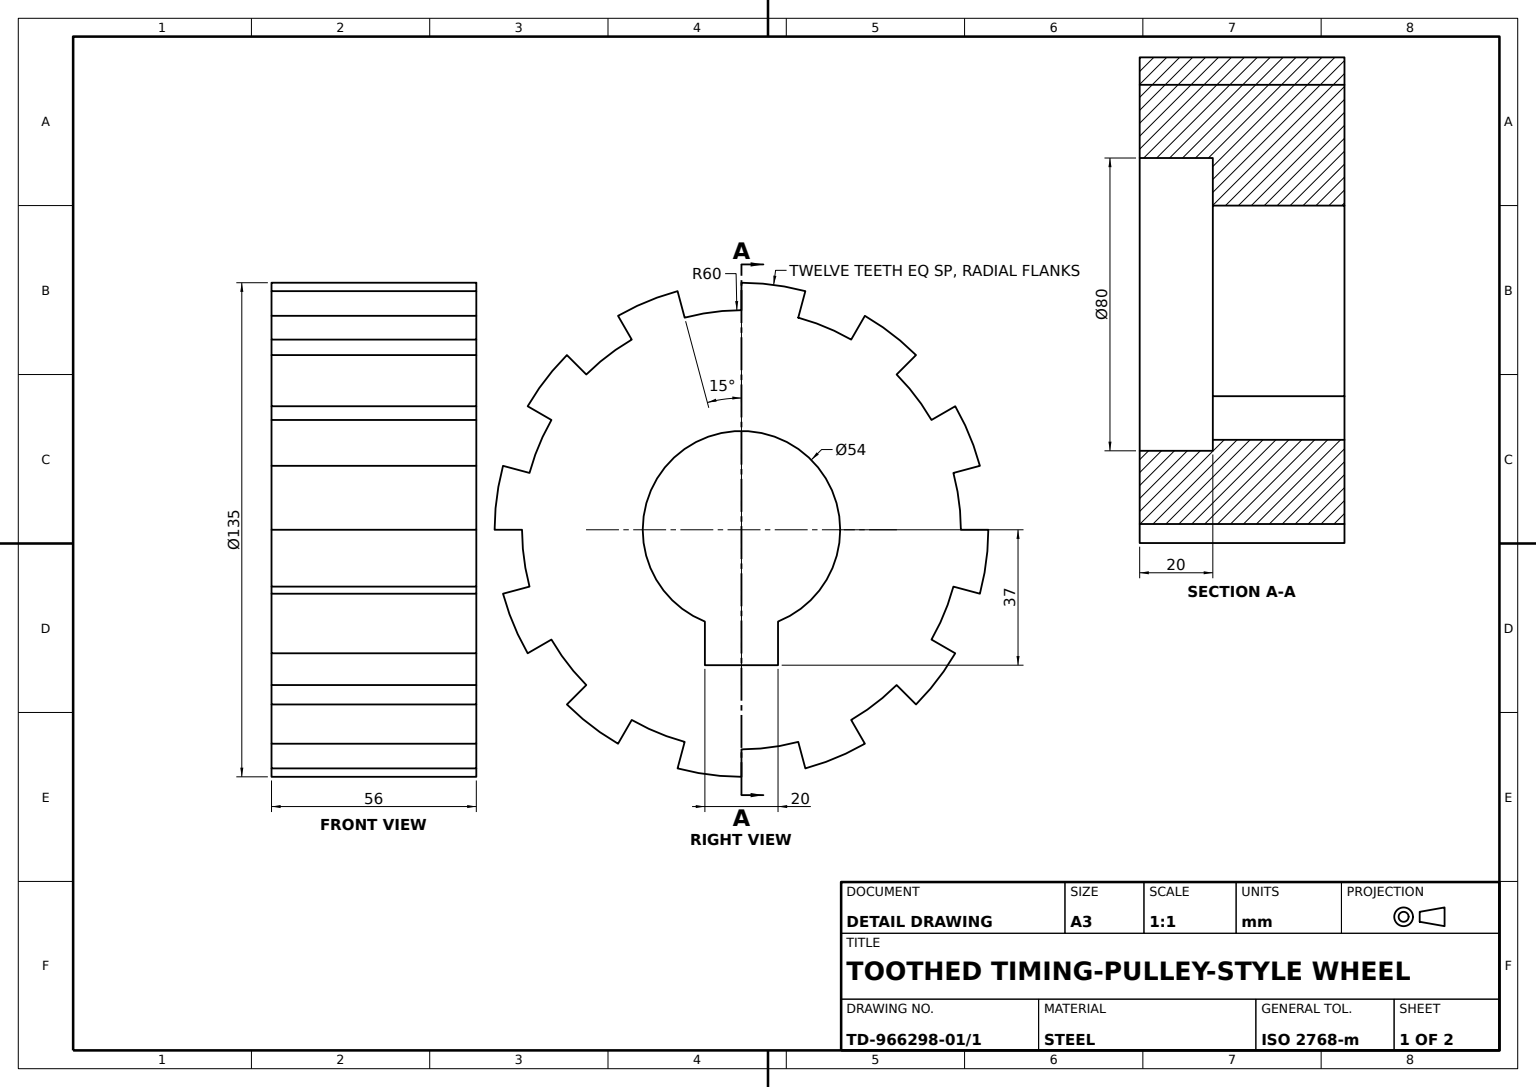
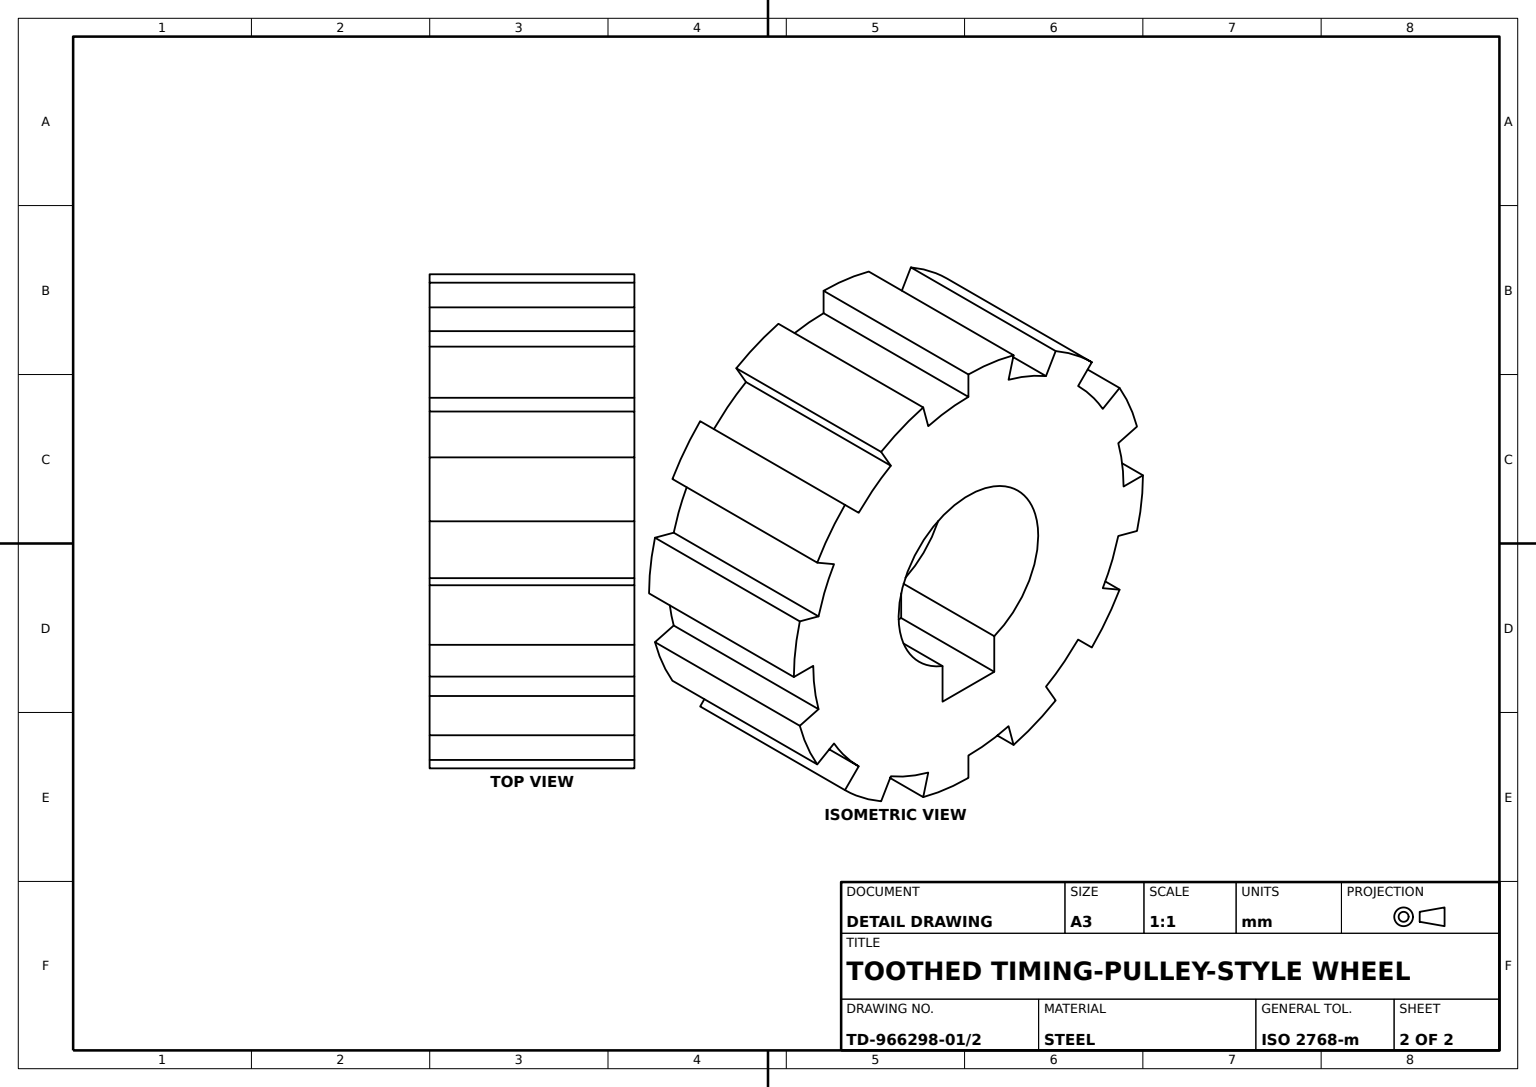
SolidWorks part; units mm, degrees
material "Plain Carbon Steel"
ref_plane "Front Plane" through (0, 0, 0) normal (0, 0, 1) x (1, 0, 0)
ref_plane "Top Plane" through (0, 0, 0) normal (0, 1, 0) x (1, 0, 0)
ref_plane "Right Plane" through (0, 0, 0) normal (1, 0, 0) x (0, 0, -1)
sketch "Gear Tooth Profile Sketch" plane through (0, 0, 0) normal (0, 0, 1) x (1, 0, 0)
  line L0 (0, 60) -> (0, 67.5)
  line L1 (42.4264, 42.4264) -> (47.7297, 47.7297)
  line L2 (30, 51.9615) -> (33.75, 58.4567)
  line L3 (15.5291, 57.9555) -> (17.4703, 65.2)
  line L4 (57.9555, 15.5291) -> (65.2, 17.4703)
  line L5 (57.9555, -15.5291) -> (65.2, -17.4703)
  line L6 (42.4264, -42.4264) -> (47.7297, -47.7297)
  line L7 (15.5291, -57.9555) -> (17.4703, -65.2)
  line L8 (-15.5291, -57.9555) -> (-17.4703, -65.2)
  line L9 (-42.4264, -42.4264) -> (-47.7297, -47.7297)
  line L10 (-57.9555, -15.5291) -> (-65.2, -17.4703)
  line L11 (-57.9555, 15.5291) -> (-65.2, 17.4703)
  line L12 (-42.4264, 42.4264) -> (-47.7297, 47.7297)
  line L13 (-15.5291, 57.9555) -> (-17.4703, 65.2)
  line L14 (51.9615, 30) -> (58.4567, 33.75)
  line L15 (60, 0) -> (67.5, 0)
  line L16 (51.9615, -30) -> (58.4567, -33.75)
  line L17 (30, -51.9615) -> (33.75, -58.4567)
  line L18 (0, -60) -> (0, -67.5)
  line L19 (-30, -51.9615) -> (-33.75, -58.4567)
  line L20 (-51.9615, -30) -> (-58.4567, -33.75)
  line L21 (-60, 0) -> (-67.5, 0)
  line L22 (-51.9615, 30) -> (-58.4567, 33.75)
  line L23 (-30, 51.9615) -> (-33.75, 58.4567)
  line L24 (0, 60) -> (0, 67.5)
  arc A0 (0, 67.5) -> (-17.4703, 65.2) centre (0, 0) ccw
  arc A1 (15.5291, 57.9555) -> (0, 60) centre (0, 0) ccw
  arc A2 (33.75, 58.4567) -> (17.4703, 65.2) centre (0, 0) ccw
  arc A3 (42.4264, 42.4264) -> (30, 51.9615) centre (0, 0) ccw
  arc A4 (58.4567, 33.75) -> (47.7297, 47.7297) centre (0, 0) ccw
  arc A5 (57.9555, 15.5291) -> (51.9615, 30) centre (0, 0) ccw
  arc A6 (67.5, 0) -> (65.2, 17.4703) centre (0, 0) ccw
  arc A7 (57.9555, -15.5291) -> (60, 0) centre (0, 0) ccw
  arc A8 (58.4567, -33.75) -> (65.2, -17.4703) centre (0, 0) ccw
  arc A9 (42.4264, -42.4264) -> (51.9615, -30) centre (0, 0) ccw
  arc A10 (33.75, -58.4567) -> (47.7297, -47.7297) centre (0, 0) ccw
  arc A11 (15.5291, -57.9555) -> (30, -51.9615) centre (0, 0) ccw
  arc A12 (0, -67.5) -> (17.4703, -65.2) centre (0, 0) ccw
  arc A13 (-15.5291, -57.9555) -> (0, -60) centre (0, 0) ccw
  arc A14 (-33.75, -58.4567) -> (-17.4703, -65.2) centre (0, 0) ccw
  arc A15 (-42.4264, -42.4264) -> (-30, -51.9615) centre (0, 0) ccw
  arc A16 (-58.4567, -33.75) -> (-47.7297, -47.7297) centre (0, 0) ccw
  arc A17 (-57.9555, -15.5291) -> (-51.9615, -30) centre (0, 0) ccw
  arc A18 (-67.5, 0) -> (-65.2, -17.4703) centre (0, 0) ccw
  arc A19 (-57.9555, 15.5291) -> (-60, 0) centre (0, 0) ccw
  arc A20 (-58.4567, 33.75) -> (-65.2, 17.4703) centre (0, 0) ccw
  arc A21 (-42.4264, 42.4264) -> (-51.9615, 30) centre (0, 0) ccw
  arc A22 (-33.75, 58.4567) -> (-47.7297, 47.7297) centre (0, 0) ccw
  arc A23 (-15.5291, 57.9555) -> (-30, 51.9615) centre (0, 0) ccw
  dimension "D1" = 67.5
  dimension "D2" = 60
  dimension "D3" = 12
  dimension "D4" = 15
  dimension "D5" = 12
  dimension "D6" = 15
  dimension "D7" = 16.2797
extrude "Gear Body 12T" add sketch "Gear Tooth Profile Sketch" against normal blind 56 contours L13 A23 L23 A22 L12 A21 L22 A20 L11 A19 L21 A18 L10 A17 L20 A16 L9 A15 L19 A14 L8 A13 L18 A12 L7 A11 L17 A10 L6 A9 L16 A8 L5 A7 L15 A6 L4 A5 L14 A4 L1 A3 L2 A2 L3 A1 L0 A0
sketch "Face Recess Sketch" plane through (0, 0, 0) normal (0, 0, 1) x (1, 0, 0)
  circle A0 centre (0, 0) radius 40
  dimension "D1" = 80
extrude "Face Recess Ø80" cut sketch "Face Recess Sketch" against normal blind 20
sketch "Bore Profile Sketch" plane through (0, 0, -20) normal (0, 0, 1) x (1, 0, 0)
  line L1 (0, -37) -> (10, -37)
  line L2 (10, -37) -> (10, -25.0799)
  line L3 (0, -37) -> (-10, -37)
  line L4 (-10, -37) -> (-10, -25.0799)
  arc A0 (10, -25.0799) -> (-10, -25.0799) centre (0, 0) ccw
  dimension "D1" = 27
  dimension "D2" = 11.9201
  dimension "D3" = 10
  dimension "D4" = 10
  dimension "D5" = 37
extrude "Bore Cut" cut sketch "Bore Profile Sketch" against normal blind 36
